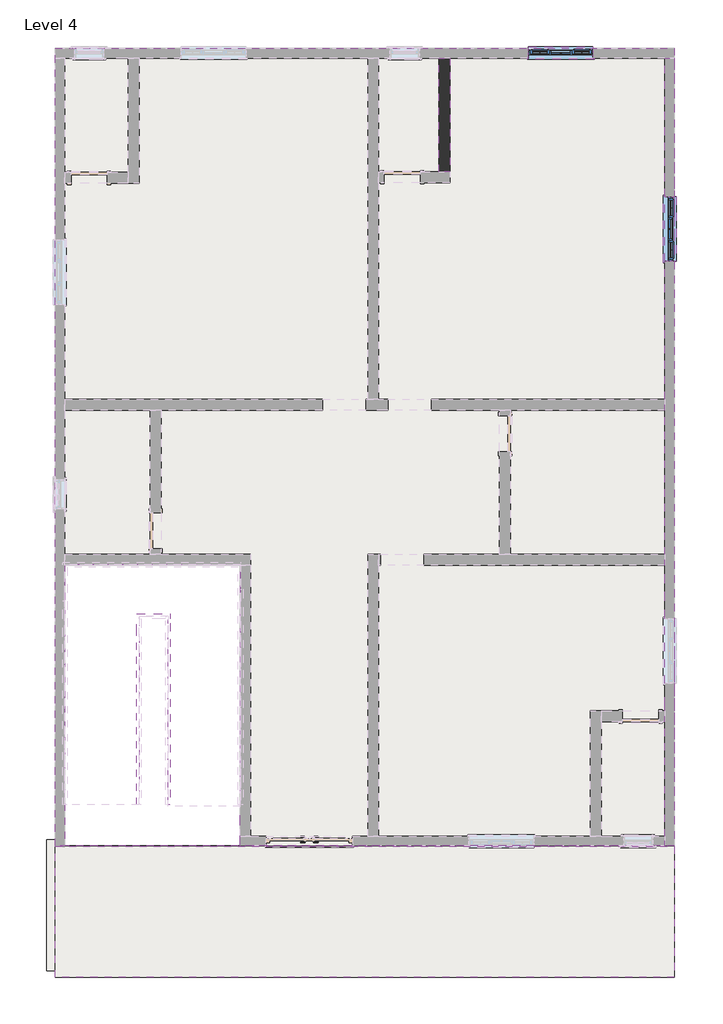
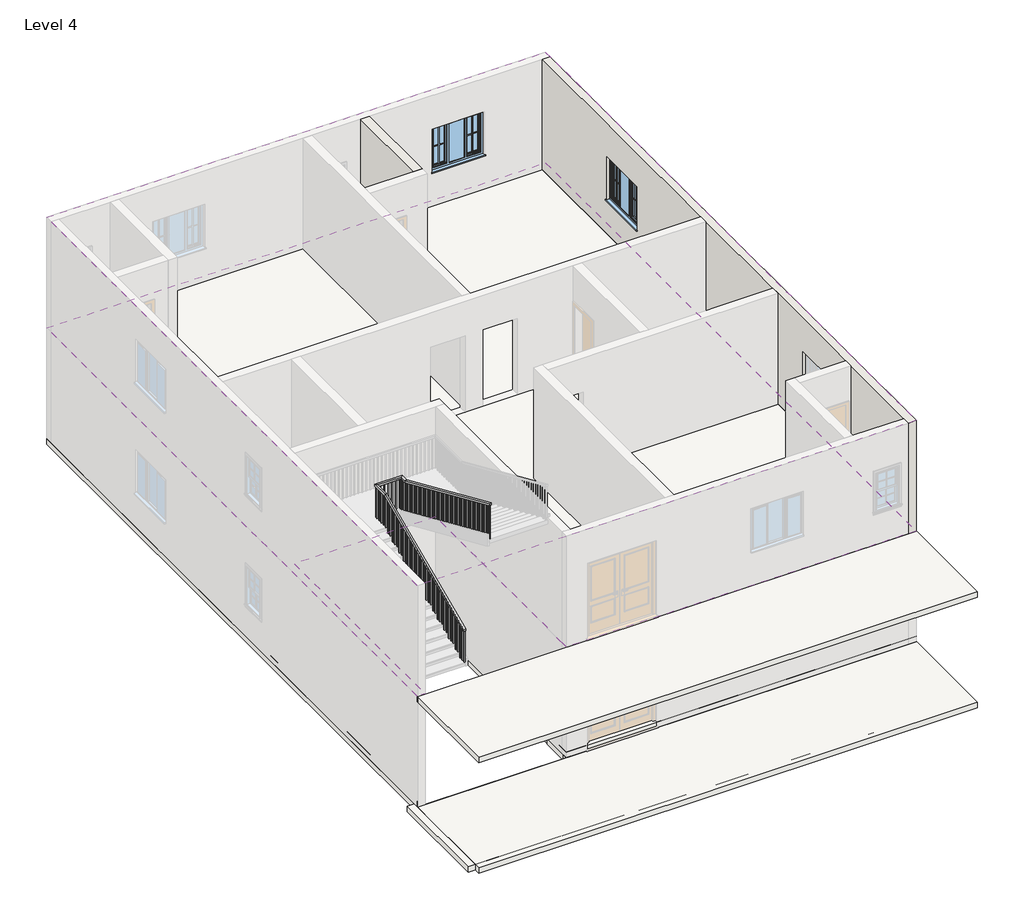
# One storey, part 3 of 5: 6 roofs, 6 slabs, 6 windows, 5 walls, 1 railing.
"""IFC4 building model written with IfcOpenShell, lengths in millimetres."""

from ifc_helpers import new_model, si_unit, frame, origin, place, context, project, spatial, polyline, outline, extrude, faceted_brep, transform, mapped, element, save
from components import windows_tpl_w_glazing_cross_bars_1360x1210mm_0306471f

model = new_model("IFC4")

# Units and contexts
model_context = context("Model", 3, world=origin())
ifc_project = project(units=[si_unit("LENGTHUNIT", "METRE", prefix="MILLI")], contexts=[model_context])

# Site, building, storey
site = spatial("IfcSite", under=ifc_project)
building = spatial("IfcBuilding", under=site)
storey = spatial("IfcBuildingStorey", under=building, Name="Level 4", Elevation=9144.0)

# Railing
placement = place(None, origin())
element("IfcRailing", 1, ObjectType="Handrail - Rectangular", at=placement, inside=storey, context=model_context, shape_type="SolidModel", body=[
    faceted_brep([(-6050.7290366, -6973.0610642, 12913.36), (-6050.7290366, -6973.0610642, 12857.8599828), (-5999.9290366, -6973.0610642, 12857.8599828), (-5999.9290366, -6973.0610642, 12913.36), (-6050.7290366, -3417.0610642, 14478.0), (-6050.7290366, -3406.3792071, 14427.2), (-5999.9290366, -3406.3792071, 14427.2), (-5999.9290366, -3417.0610642, 14478.0), (-6050.7290366, -2959.8610642, 14478.0), (-6050.7290366, -2959.8610642, 14427.2), (-5999.9290366, -3010.6610642, 14427.2), (-5999.9290366, -3010.6610642, 14478.0), (-5339.5290366, -2959.8610642, 14478.0), (-5339.5290366, -2959.8610642, 14427.2), (-5390.3290366, -3010.6610642, 14427.2), (-5390.3290366, -3010.6610642, 14478.0), (-5339.5290366, -3163.0610642, 14478.0), (-5339.5290366, -3173.7429214, 14427.2), (-5390.3290366, -3173.7429214, 14427.2), (-5390.3290366, -3163.0610642, 14478.0), (-5339.5290366, -6973.0610642, 16154.4), (-5390.3290366, -6973.0610642, 16154.4), (-5390.3290366, -6973.0610642, 16098.8999828), (-5339.5290366, -6973.0610642, 16098.8999828)], [[[0, 1, 2, 3]], [[1, 0, 4, 5]], [[2, 1, 5, 6]], [[3, 2, 6, 7]], [[0, 3, 7, 4]], [[5, 4, 8, 9]], [[6, 5, 9, 10]], [[7, 6, 10, 11]], [[4, 7, 11, 8]], [[9, 8, 12, 13]], [[10, 9, 13, 14]], [[11, 10, 14, 15]], [[8, 11, 15, 12]], [[13, 12, 16, 17]], [[14, 13, 17, 18]], [[15, 14, 18, 19]], [[12, 15, 19, 16]], [[20, 21, 22, 23]], [[17, 16, 20, 23]], [[18, 17, 23, 22]], [[19, 18, 22, 21]], [[16, 19, 21, 20]]]),
    extrude(outline(polyline([(-6957.1860642, 16091.9149828), (-6938.1360642, 16083.5329828), (-6938.1360642, 15128.24), (-6957.1860642, 15128.24), (-6957.1860642, 16091.9149828)])), frame((-5374.4540366, 0.0, 0.0), z_axis=(1.0, 0.0, 0.0), x_axis=(0.0, 1.0, 0.0)), (0.0, 0.0, 1.0), 19.05),
    extrude(outline(polyline([(-6855.5860642, 16047.2109828), (-6836.5360642, 16038.8289828), (-6836.5360642, 15128.24), (-6855.5860642, 15128.24), (-6855.5860642, 16047.2109828)])), frame((-5374.4540366, 0.0, 0.0), z_axis=(1.0, 0.0, 0.0), x_axis=(0.0, 1.0, 0.0)), (0.0, 0.0, 1.0), 19.05),
    extrude(outline(polyline([(-6753.9860642, 16002.5069828), (-6734.9360642, 15994.1249828), (-6734.9360642, 15128.24), (-6753.9860642, 15128.24), (-6753.9860642, 16002.5069828)])), frame((-5374.4540366, 0.0, 0.0), z_axis=(1.0, 0.0, 0.0), x_axis=(0.0, 1.0, 0.0)), (0.0, 0.0, 1.0), 19.05),
    extrude(outline(polyline([(-6652.3860642, 15957.8029828), (-6633.3360642, 15949.4209828), (-6633.3360642, 15016.48), (-6652.3860642, 15016.48), (-6652.3860642, 15957.8029828)])), frame((-5374.4540366, 0.0, 0.0), z_axis=(1.0, 0.0, 0.0), x_axis=(0.0, 1.0, 0.0)), (0.0, 0.0, 1.0), 19.05),
    extrude(outline(polyline([(-6550.7860642, 15913.0989828), (-6531.7360642, 15904.7169828), (-6531.7360642, 15016.48), (-6550.7860642, 15016.48), (-6550.7860642, 15913.0989828)])), frame((-5374.4540366, 0.0, 0.0), z_axis=(1.0, 0.0, 0.0), x_axis=(0.0, 1.0, 0.0)), (0.0, 0.0, 1.0), 19.05),
    extrude(outline(polyline([(-6449.1860642, 15868.3949828), (-6430.1360642, 15860.0129828), (-6430.1360642, 14904.72), (-6449.1860642, 14904.72), (-6449.1860642, 15868.3949828)])), frame((-5374.4540366, 0.0, 0.0), z_axis=(1.0, 0.0, 0.0), x_axis=(0.0, 1.0, 0.0)), (0.0, 0.0, 1.0), 19.05),
    extrude(outline(polyline([(-6347.5860642, 15823.6909828), (-6328.5360642, 15815.3089828), (-6328.5360642, 14904.72), (-6347.5860642, 14904.72), (-6347.5860642, 15823.6909828)])), frame((-5374.4540366, 0.0, 0.0), z_axis=(1.0, 0.0, 0.0), x_axis=(0.0, 1.0, 0.0)), (0.0, 0.0, 1.0), 19.05),
    extrude(outline(polyline([(-6245.9860642, 15778.9869828), (-6226.9360642, 15770.6049828), (-6226.9360642, 14904.72), (-6245.9860642, 14904.72), (-6245.9860642, 15778.9869828)])), frame((-5374.4540366, 0.0, 0.0), z_axis=(1.0, 0.0, 0.0), x_axis=(0.0, 1.0, 0.0)), (0.0, 0.0, 1.0), 19.05),
    extrude(outline(polyline([(-6144.3860642, 15734.2829828), (-6125.3360642, 15725.9009828), (-6125.3360642, 14792.96), (-6144.3860642, 14792.96), (-6144.3860642, 15734.2829828)])), frame((-5374.4540366, 0.0, 0.0), z_axis=(1.0, 0.0, 0.0), x_axis=(0.0, 1.0, 0.0)), (0.0, 0.0, 1.0), 19.05),
    extrude(outline(polyline([(-6042.7860642, 15689.5789828), (-6023.7360642, 15681.1969828), (-6023.7360642, 14792.96), (-6042.7860642, 14792.96), (-6042.7860642, 15689.5789828)])), frame((-5374.4540366, 0.0, 0.0), z_axis=(1.0, 0.0, 0.0), x_axis=(0.0, 1.0, 0.0)), (0.0, 0.0, 1.0), 19.05),
    extrude(outline(polyline([(-5941.1860642, 15644.8749828), (-5922.1360642, 15636.4929828), (-5922.1360642, 14681.2), (-5941.1860642, 14681.2), (-5941.1860642, 15644.8749828)])), frame((-5374.4540366, 0.0, 0.0), z_axis=(1.0, 0.0, 0.0), x_axis=(0.0, 1.0, 0.0)), (0.0, 0.0, 1.0), 19.05),
    extrude(outline(polyline([(-5839.5860642, 15600.1709828), (-5820.5360642, 15591.7889828), (-5820.5360642, 14681.2), (-5839.5860642, 14681.2), (-5839.5860642, 15600.1709828)])), frame((-5374.4540366, 0.0, 0.0), z_axis=(1.0, 0.0, 0.0), x_axis=(0.0, 1.0, 0.0)), (0.0, 0.0, 1.0), 19.05),
    extrude(outline(polyline([(-5737.9860642, 15555.4669828), (-5718.9360642, 15547.0849828), (-5718.9360642, 14681.2), (-5737.9860642, 14681.2), (-5737.9860642, 15555.4669828)])), frame((-5374.4540366, 0.0, 0.0), z_axis=(1.0, 0.0, 0.0), x_axis=(0.0, 1.0, 0.0)), (0.0, 0.0, 1.0), 19.05),
    extrude(outline(polyline([(-5636.3860642, 15510.7629828), (-5617.3360642, 15502.3809828), (-5617.3360642, 14569.44), (-5636.3860642, 14569.44), (-5636.3860642, 15510.7629828)])), frame((-5374.4540366, 0.0, 0.0), z_axis=(1.0, 0.0, 0.0), x_axis=(0.0, 1.0, 0.0)), (0.0, 0.0, 1.0), 19.05),
    extrude(outline(polyline([(-5534.7860642, 15466.0589828), (-5515.7360642, 15457.6769828), (-5515.7360642, 14569.44), (-5534.7860642, 14569.44), (-5534.7860642, 15466.0589828)])), frame((-5374.4540366, 0.0, 0.0), z_axis=(1.0, 0.0, 0.0), x_axis=(0.0, 1.0, 0.0)), (0.0, 0.0, 1.0), 19.05),
    extrude(outline(polyline([(-5433.1860642, 15421.3549828), (-5414.1360642, 15412.9729828), (-5414.1360642, 14457.68), (-5433.1860642, 14457.68), (-5433.1860642, 15421.3549828)])), frame((-5374.4540366, 0.0, 0.0), z_axis=(1.0, 0.0, 0.0), x_axis=(0.0, 1.0, 0.0)), (0.0, 0.0, 1.0), 19.05),
    extrude(outline(polyline([(-5331.5860642, 15376.6509828), (-5312.5360642, 15368.2689828), (-5312.5360642, 14457.68), (-5331.5860642, 14457.68), (-5331.5860642, 15376.6509828)])), frame((-5374.4540366, 0.0, 0.0), z_axis=(1.0, 0.0, 0.0), x_axis=(0.0, 1.0, 0.0)), (0.0, 0.0, 1.0), 19.05),
    extrude(outline(polyline([(-5229.9860642, 15331.9469828), (-5210.9360642, 15323.5649828), (-5210.9360642, 14457.68), (-5229.9860642, 14457.68), (-5229.9860642, 15331.9469828)])), frame((-5374.4540366, 0.0, 0.0), z_axis=(1.0, 0.0, 0.0), x_axis=(0.0, 1.0, 0.0)), (0.0, 0.0, 1.0), 19.05),
    extrude(outline(polyline([(-5128.3860642, 15287.2429828), (-5109.3360642, 15278.8609828), (-5109.3360642, 14345.92), (-5128.3860642, 14345.92), (-5128.3860642, 15287.2429828)])), frame((-5374.4540366, 0.0, 0.0), z_axis=(1.0, 0.0, 0.0), x_axis=(0.0, 1.0, 0.0)), (0.0, 0.0, 1.0), 19.05),
    extrude(outline(polyline([(-5026.7860642, 15242.5389828), (-5007.7360642, 15234.1569828), (-5007.7360642, 14345.92), (-5026.7860642, 14345.92), (-5026.7860642, 15242.5389828)])), frame((-5374.4540366, 0.0, 0.0), z_axis=(1.0, 0.0, 0.0), x_axis=(0.0, 1.0, 0.0)), (0.0, 0.0, 1.0), 19.05),
    extrude(outline(polyline([(-4925.1860642, 15197.8349828), (-4906.1360642, 15189.4529828), (-4906.1360642, 14234.16), (-4925.1860642, 14234.16), (-4925.1860642, 15197.8349828)])), frame((-5374.4540366, 0.0, 0.0), z_axis=(1.0, 0.0, 0.0), x_axis=(0.0, 1.0, 0.0)), (0.0, 0.0, 1.0), 19.05),
    extrude(outline(polyline([(-4823.5860642, 15153.1309828), (-4804.5360642, 15144.7489828), (-4804.5360642, 14234.16), (-4823.5860642, 14234.16), (-4823.5860642, 15153.1309828)])), frame((-5374.4540366, 0.0, 0.0), z_axis=(1.0, 0.0, 0.0), x_axis=(0.0, 1.0, 0.0)), (0.0, 0.0, 1.0), 19.05),
    extrude(outline(polyline([(-4721.9860642, 15108.4269828), (-4702.9360642, 15100.0449828), (-4702.9360642, 14234.16), (-4721.9860642, 14234.16), (-4721.9860642, 15108.4269828)])), frame((-5374.4540366, 0.0, 0.0), z_axis=(1.0, 0.0, 0.0), x_axis=(0.0, 1.0, 0.0)), (0.0, 0.0, 1.0), 19.05),
    extrude(outline(polyline([(-4620.3860642, 15063.7229828), (-4601.3360642, 15055.3409828), (-4601.3360642, 14122.4), (-4620.3860642, 14122.4), (-4620.3860642, 15063.7229828)])), frame((-5374.4540366, 0.0, 0.0), z_axis=(1.0, 0.0, 0.0), x_axis=(0.0, 1.0, 0.0)), (0.0, 0.0, 1.0), 19.05),
    extrude(outline(polyline([(-4518.7860642, 15019.0189828), (-4499.7360642, 15010.6369828), (-4499.7360642, 14122.4), (-4518.7860642, 14122.4), (-4518.7860642, 15019.0189828)])), frame((-5374.4540366, 0.0, 0.0), z_axis=(1.0, 0.0, 0.0), x_axis=(0.0, 1.0, 0.0)), (0.0, 0.0, 1.0), 19.05),
    extrude(outline(polyline([(-4417.1860642, 14974.3149828), (-4398.1360642, 14965.9329828), (-4398.1360642, 14010.64), (-4417.1860642, 14010.64), (-4417.1860642, 14974.3149828)])), frame((-5374.4540366, 0.0, 0.0), z_axis=(1.0, 0.0, 0.0), x_axis=(0.0, 1.0, 0.0)), (0.0, 0.0, 1.0), 19.05),
    extrude(outline(polyline([(-4315.5860642, 14929.6109828), (-4296.5360642, 14921.2289828), (-4296.5360642, 14010.64), (-4315.5860642, 14010.64), (-4315.5860642, 14929.6109828)])), frame((-5374.4540366, 0.0, 0.0), z_axis=(1.0, 0.0, 0.0), x_axis=(0.0, 1.0, 0.0)), (0.0, 0.0, 1.0), 19.05),
    extrude(outline(polyline([(-4213.9860642, 14884.9069828), (-4194.9360642, 14876.5249828), (-4194.9360642, 14010.64), (-4213.9860642, 14010.64), (-4213.9860642, 14884.9069828)])), frame((-5374.4540366, 0.0, 0.0), z_axis=(1.0, 0.0, 0.0), x_axis=(0.0, 1.0, 0.0)), (0.0, 0.0, 1.0), 19.05),
    extrude(outline(polyline([(-4112.3860642, 14840.2029828), (-4093.3360642, 14831.8209828), (-4093.3360642, 13898.88), (-4112.3860642, 13898.88), (-4112.3860642, 14840.2029828)])), frame((-5374.4540366, 0.0, 0.0), z_axis=(1.0, 0.0, 0.0), x_axis=(0.0, 1.0, 0.0)), (0.0, 0.0, 1.0), 19.05),
    extrude(outline(polyline([(-4010.7860642, 14795.4989828), (-3991.7360642, 14787.1169828), (-3991.7360642, 13898.88), (-4010.7860642, 13898.88), (-4010.7860642, 14795.4989828)])), frame((-5374.4540366, 0.0, 0.0), z_axis=(1.0, 0.0, 0.0), x_axis=(0.0, 1.0, 0.0)), (0.0, 0.0, 1.0), 19.05),
    extrude(outline(polyline([(-3909.1860642, 14750.7949828), (-3890.1360642, 14742.4129828), (-3890.1360642, 13787.12), (-3909.1860642, 13787.12), (-3909.1860642, 14750.7949828)])), frame((-5374.4540366, 0.0, 0.0), z_axis=(1.0, 0.0, 0.0), x_axis=(0.0, 1.0, 0.0)), (0.0, 0.0, 1.0), 19.05),
    extrude(outline(polyline([(-3807.5860642, 14706.0909828), (-3788.5360642, 14697.7089828), (-3788.5360642, 13787.12), (-3807.5860642, 13787.12), (-3807.5860642, 14706.0909828)])), frame((-5374.4540366, 0.0, 0.0), z_axis=(1.0, 0.0, 0.0), x_axis=(0.0, 1.0, 0.0)), (0.0, 0.0, 1.0), 19.05),
    extrude(outline(polyline([(-3705.9860642, 14661.3869828), (-3686.9360642, 14653.0049828), (-3686.9360642, 13787.12), (-3705.9860642, 13787.12), (-3705.9860642, 14661.3869828)])), frame((-5374.4540366, 0.0, 0.0), z_axis=(1.0, 0.0, 0.0), x_axis=(0.0, 1.0, 0.0)), (0.0, 0.0, 1.0), 19.05),
    extrude(outline(polyline([(-3604.3860642, 14616.6829828), (-3585.3360642, 14608.3009828), (-3585.3360642, 13675.36), (-3604.3860642, 13675.36), (-3604.3860642, 14616.6829828)])), frame((-5374.4540366, 0.0, 0.0), z_axis=(1.0, 0.0, 0.0), x_axis=(0.0, 1.0, 0.0)), (0.0, 0.0, 1.0), 19.05),
    extrude(outline(polyline([(-3502.7860642, 14571.9789828), (-3483.7360642, 14563.5969828), (-3483.7360642, 13675.36), (-3502.7860642, 13675.36), (-3502.7860642, 14571.9789828)])), frame((-5374.4540366, 0.0, 0.0), z_axis=(1.0, 0.0, 0.0), x_axis=(0.0, 1.0, 0.0)), (0.0, 0.0, 1.0), 19.05),
    extrude(outline(polyline([(-3401.1860642, 14527.2749828), (-3382.1360642, 14518.8929828), (-3382.1360642, 13563.6), (-3401.1860642, 13563.6), (-3401.1860642, 14527.2749828)])), frame((-5374.4540366, 0.0, 0.0), z_axis=(1.0, 0.0, 0.0), x_axis=(0.0, 1.0, 0.0)), (0.0, 0.0, 1.0), 19.05),
    extrude(outline(polyline([(-3299.5860642, 14482.5709828), (-3280.5360642, 14474.1889828), (-3280.5360642, 13563.6), (-3299.5860642, 13563.6), (-3299.5860642, 14482.5709828)])), frame((-5374.4540366, 0.0, 0.0), z_axis=(1.0, 0.0, 0.0), x_axis=(0.0, 1.0, 0.0)), (0.0, 0.0, 1.0), 19.05),
    extrude(outline(polyline([(-3197.9860642, 14437.8669828), (-3178.9360642, 14429.4849828), (-3178.9360642, 13563.6), (-3197.9860642, 13563.6), (-3197.9860642, 14437.8669828)])), frame((-5374.4540366, 0.0, 0.0), z_axis=(1.0, 0.0, 0.0), x_axis=(0.0, 1.0, 0.0)), (0.0, 0.0, 1.0), 19.05),
    extrude(outline(polyline([(-5374.4540366, -3077.3360642), (-5355.4040366, -3077.3360642), (-5355.4040366, -3096.3860642), (-5374.4540366, -3096.3860642), (-5374.4540366, -3077.3360642)])), frame((0.0, 0.0, 13563.6), z_axis=(0.0, 0.0, 1.0), x_axis=(1.0, 0.0, 0.0)), (0.0, 0.0, 1.0), 863.6),
    extrude(outline(polyline([(-5425.2540366, -2994.7860642), (-5425.2540366, -2975.7360642), (-5406.2040366, -2975.7360642), (-5406.2040366, -2994.7860642), (-5425.2540366, -2994.7860642)])), frame((0.0, 0.0, 13563.6), z_axis=(0.0, 0.0, 1.0), x_axis=(1.0, 0.0, 0.0)), (0.0, 0.0, 1.0), 863.6),
    extrude(outline(polyline([(-5526.8540366, -2994.7860642), (-5526.8540366, -2975.7360642), (-5507.8040366, -2975.7360642), (-5507.8040366, -2994.7860642), (-5526.8540366, -2994.7860642)])), frame((0.0, 0.0, 13563.6), z_axis=(0.0, 0.0, 1.0), x_axis=(1.0, 0.0, 0.0)), (0.0, 0.0, 1.0), 863.6),
    extrude(outline(polyline([(-5628.4540366, -2994.7860642), (-5628.4540366, -2975.7360642), (-5609.4040366, -2975.7360642), (-5609.4040366, -2994.7860642), (-5628.4540366, -2994.7860642)])), frame((0.0, 0.0, 13563.6), z_axis=(0.0, 0.0, 1.0), x_axis=(1.0, 0.0, 0.0)), (0.0, 0.0, 1.0), 863.6),
    extrude(outline(polyline([(-5730.0540366, -2994.7860642), (-5730.0540366, -2975.7360642), (-5711.0040366, -2975.7360642), (-5711.0040366, -2994.7860642), (-5730.0540366, -2994.7860642)])), frame((0.0, 0.0, 13563.6), z_axis=(0.0, 0.0, 1.0), x_axis=(1.0, 0.0, 0.0)), (0.0, 0.0, 1.0), 863.6),
    extrude(outline(polyline([(-5831.6540366, -2994.7860642), (-5831.6540366, -2975.7360642), (-5812.6040366, -2975.7360642), (-5812.6040366, -2994.7860642), (-5831.6540366, -2994.7860642)])), frame((0.0, 0.0, 13563.6), z_axis=(0.0, 0.0, 1.0), x_axis=(1.0, 0.0, 0.0)), (0.0, 0.0, 1.0), 863.6),
    extrude(outline(polyline([(-5933.2540366, -2994.7860642), (-5933.2540366, -2975.7360642), (-5914.2040366, -2975.7360642), (-5914.2040366, -2994.7860642), (-5933.2540366, -2994.7860642)])), frame((0.0, 0.0, 13563.6), z_axis=(0.0, 0.0, 1.0), x_axis=(1.0, 0.0, 0.0)), (0.0, 0.0, 1.0), 863.6),
    extrude(outline(polyline([(-6015.8040366, -3020.1860642), (-6034.8540366, -3020.1860642), (-6034.8540366, -3001.1360642), (-6015.8040366, -3001.1360642), (-6015.8040366, -3020.1860642)])), frame((0.0, 0.0, 13563.6), z_axis=(0.0, 0.0, 1.0), x_axis=(1.0, 0.0, 0.0)), (0.0, 0.0, 1.0), 863.6),
    extrude(outline(polyline([(-6015.8040366, -3121.7860642), (-6034.8540366, -3121.7860642), (-6034.8540366, -3102.7360642), (-6015.8040366, -3102.7360642), (-6015.8040366, -3121.7860642)])), frame((0.0, 0.0, 13563.6), z_axis=(0.0, 0.0, 1.0), x_axis=(1.0, 0.0, 0.0)), (0.0, 0.0, 1.0), 863.6),
    extrude(outline(polyline([(-6015.8040366, -3223.3860642), (-6034.8540366, -3223.3860642), (-6034.8540366, -3204.3360642), (-6015.8040366, -3204.3360642), (-6015.8040366, -3223.3860642)])), frame((0.0, 0.0, 13563.6), z_axis=(0.0, 0.0, 1.0), x_axis=(1.0, 0.0, 0.0)), (0.0, 0.0, 1.0), 863.6),
    extrude(outline(polyline([(-6015.8040366, -3324.9860642), (-6034.8540366, -3324.9860642), (-6034.8540366, -3305.9360642), (-6015.8040366, -3305.9360642), (-6015.8040366, -3324.9860642)])), frame((0.0, 0.0, 13563.6), z_axis=(0.0, 0.0, 1.0), x_axis=(1.0, 0.0, 0.0)), (0.0, 0.0, 1.0), 863.6),
    extrude(outline(polyline([(-3426.5860642, 14418.3089828), (-3407.5360642, 14426.6909828), (-3407.5360642, 13563.6), (-3426.5860642, 13563.6), (-3426.5860642, 14418.3089828)])), frame((-6034.8540366, 0.0, 0.0), z_axis=(1.0, 0.0, 0.0), x_axis=(0.0, 1.0, 0.0)), (0.0, 0.0, 1.0), 19.05),
    extrude(outline(polyline([(-3528.1860642, 14373.6049828), (-3509.1360642, 14381.9869828), (-3509.1360642, 13451.84), (-3528.1860642, 13451.84), (-3528.1860642, 14373.6049828)])), frame((-6034.8540366, 0.0, 0.0), z_axis=(1.0, 0.0, 0.0), x_axis=(0.0, 1.0, 0.0)), (0.0, 0.0, 1.0), 19.05),
    extrude(outline(polyline([(-3629.7860642, 14328.9009828), (-3610.7360642, 14337.2829828), (-3610.7360642, 13451.84), (-3629.7860642, 13451.84), (-3629.7860642, 14328.9009828)])), frame((-6034.8540366, 0.0, 0.0), z_axis=(1.0, 0.0, 0.0), x_axis=(0.0, 1.0, 0.0)), (0.0, 0.0, 1.0), 19.05),
    extrude(outline(polyline([(-3731.3860642, 14284.1969828), (-3712.3360642, 14292.5789828), (-3712.3360642, 13340.08), (-3731.3860642, 13340.08), (-3731.3860642, 14284.1969828)])), frame((-6034.8540366, 0.0, 0.0), z_axis=(1.0, 0.0, 0.0), x_axis=(0.0, 1.0, 0.0)), (0.0, 0.0, 1.0), 19.05),
    extrude(outline(polyline([(-3832.9860642, 14239.4929828), (-3813.9360642, 14247.8749828), (-3813.9360642, 13340.08), (-3832.9860642, 13340.08), (-3832.9860642, 14239.4929828)])), frame((-6034.8540366, 0.0, 0.0), z_axis=(1.0, 0.0, 0.0), x_axis=(0.0, 1.0, 0.0)), (0.0, 0.0, 1.0), 19.05),
    extrude(outline(polyline([(-3934.5860642, 14194.7889828), (-3915.5360642, 14203.1709828), (-3915.5360642, 13340.08), (-3934.5860642, 13340.08), (-3934.5860642, 14194.7889828)])), frame((-6034.8540366, 0.0, 0.0), z_axis=(1.0, 0.0, 0.0), x_axis=(0.0, 1.0, 0.0)), (0.0, 0.0, 1.0), 19.05),
    extrude(outline(polyline([(-4036.1860642, 14150.0849828), (-4017.1360642, 14158.4669828), (-4017.1360642, 13228.32), (-4036.1860642, 13228.32), (-4036.1860642, 14150.0849828)])), frame((-6034.8540366, 0.0, 0.0), z_axis=(1.0, 0.0, 0.0), x_axis=(0.0, 1.0, 0.0)), (0.0, 0.0, 1.0), 19.05),
    extrude(outline(polyline([(-4137.7860642, 14105.3809828), (-4118.7360642, 14113.7629828), (-4118.7360642, 13228.32), (-4137.7860642, 13228.32), (-4137.7860642, 14105.3809828)])), frame((-6034.8540366, 0.0, 0.0), z_axis=(1.0, 0.0, 0.0), x_axis=(0.0, 1.0, 0.0)), (0.0, 0.0, 1.0), 19.05),
    extrude(outline(polyline([(-4239.3860642, 14060.6769828), (-4220.3360642, 14069.0589828), (-4220.3360642, 13116.56), (-4239.3860642, 13116.56), (-4239.3860642, 14060.6769828)])), frame((-6034.8540366, 0.0, 0.0), z_axis=(1.0, 0.0, 0.0), x_axis=(0.0, 1.0, 0.0)), (0.0, 0.0, 1.0), 19.05),
    extrude(outline(polyline([(-4340.9860642, 14015.9729828), (-4321.9360642, 14024.3549828), (-4321.9360642, 13116.56), (-4340.9860642, 13116.56), (-4340.9860642, 14015.9729828)])), frame((-6034.8540366, 0.0, 0.0), z_axis=(1.0, 0.0, 0.0), x_axis=(0.0, 1.0, 0.0)), (0.0, 0.0, 1.0), 19.05),
    extrude(outline(polyline([(-4442.5860642, 13971.2689828), (-4423.5360642, 13979.6509828), (-4423.5360642, 13116.56), (-4442.5860642, 13116.56), (-4442.5860642, 13971.2689828)])), frame((-6034.8540366, 0.0, 0.0), z_axis=(1.0, 0.0, 0.0), x_axis=(0.0, 1.0, 0.0)), (0.0, 0.0, 1.0), 19.05),
    extrude(outline(polyline([(-4544.1860642, 13926.5649828), (-4525.1360642, 13934.9469828), (-4525.1360642, 13004.8), (-4544.1860642, 13004.8), (-4544.1860642, 13926.5649828)])), frame((-6034.8540366, 0.0, 0.0), z_axis=(1.0, 0.0, 0.0), x_axis=(0.0, 1.0, 0.0)), (0.0, 0.0, 1.0), 19.05),
    extrude(outline(polyline([(-4645.7860642, 13881.8609828), (-4626.7360642, 13890.2429828), (-4626.7360642, 13004.8), (-4645.7860642, 13004.8), (-4645.7860642, 13881.8609828)])), frame((-6034.8540366, 0.0, 0.0), z_axis=(1.0, 0.0, 0.0), x_axis=(0.0, 1.0, 0.0)), (0.0, 0.0, 1.0), 19.05),
    extrude(outline(polyline([(-4747.3860642, 13837.1569828), (-4728.3360642, 13845.5389828), (-4728.3360642, 12893.04), (-4747.3860642, 12893.04), (-4747.3860642, 13837.1569828)])), frame((-6034.8540366, 0.0, 0.0), z_axis=(1.0, 0.0, 0.0), x_axis=(0.0, 1.0, 0.0)), (0.0, 0.0, 1.0), 19.05),
    extrude(outline(polyline([(-4848.9860642, 13792.4529828), (-4829.9360642, 13800.8349828), (-4829.9360642, 12893.04), (-4848.9860642, 12893.04), (-4848.9860642, 13792.4529828)])), frame((-6034.8540366, 0.0, 0.0), z_axis=(1.0, 0.0, 0.0), x_axis=(0.0, 1.0, 0.0)), (0.0, 0.0, 1.0), 19.05),
    extrude(outline(polyline([(-4950.5860642, 13747.7489828), (-4931.5360642, 13756.1309828), (-4931.5360642, 12893.04), (-4950.5860642, 12893.04), (-4950.5860642, 13747.7489828)])), frame((-6034.8540366, 0.0, 0.0), z_axis=(1.0, 0.0, 0.0), x_axis=(0.0, 1.0, 0.0)), (0.0, 0.0, 1.0), 19.05),
    extrude(outline(polyline([(-5052.1860642, 13703.0449828), (-5033.1360642, 13711.4269828), (-5033.1360642, 12781.28), (-5052.1860642, 12781.28), (-5052.1860642, 13703.0449828)])), frame((-6034.8540366, 0.0, 0.0), z_axis=(1.0, 0.0, 0.0), x_axis=(0.0, 1.0, 0.0)), (0.0, 0.0, 1.0), 19.05),
    extrude(outline(polyline([(-5153.7860642, 13658.3409828), (-5134.7360642, 13666.7229828), (-5134.7360642, 12781.28), (-5153.7860642, 12781.28), (-5153.7860642, 13658.3409828)])), frame((-6034.8540366, 0.0, 0.0), z_axis=(1.0, 0.0, 0.0), x_axis=(0.0, 1.0, 0.0)), (0.0, 0.0, 1.0), 19.05),
    extrude(outline(polyline([(-5255.3860642, 13613.6369828), (-5236.3360642, 13622.0189828), (-5236.3360642, 12669.52), (-5255.3860642, 12669.52), (-5255.3860642, 13613.6369828)])), frame((-6034.8540366, 0.0, 0.0), z_axis=(1.0, 0.0, 0.0), x_axis=(0.0, 1.0, 0.0)), (0.0, 0.0, 1.0), 19.05),
    extrude(outline(polyline([(-5356.9860642, 13568.9329828), (-5337.9360642, 13577.3149828), (-5337.9360642, 12669.52), (-5356.9860642, 12669.52), (-5356.9860642, 13568.9329828)])), frame((-6034.8540366, 0.0, 0.0), z_axis=(1.0, 0.0, 0.0), x_axis=(0.0, 1.0, 0.0)), (0.0, 0.0, 1.0), 19.05),
    extrude(outline(polyline([(-5458.5860642, 13524.2289828), (-5439.5360642, 13532.6109828), (-5439.5360642, 12669.52), (-5458.5860642, 12669.52), (-5458.5860642, 13524.2289828)])), frame((-6034.8540366, 0.0, 0.0), z_axis=(1.0, 0.0, 0.0), x_axis=(0.0, 1.0, 0.0)), (0.0, 0.0, 1.0), 19.05),
    extrude(outline(polyline([(-5560.1860642, 13479.5249828), (-5541.1360642, 13487.9069828), (-5541.1360642, 12557.76), (-5560.1860642, 12557.76), (-5560.1860642, 13479.5249828)])), frame((-6034.8540366, 0.0, 0.0), z_axis=(1.0, 0.0, 0.0), x_axis=(0.0, 1.0, 0.0)), (0.0, 0.0, 1.0), 19.05),
    extrude(outline(polyline([(-5661.7860642, 13434.8209828), (-5642.7360642, 13443.2029828), (-5642.7360642, 12557.76), (-5661.7860642, 12557.76), (-5661.7860642, 13434.8209828)])), frame((-6034.8540366, 0.0, 0.0), z_axis=(1.0, 0.0, 0.0), x_axis=(0.0, 1.0, 0.0)), (0.0, 0.0, 1.0), 19.05),
    extrude(outline(polyline([(-5763.3860642, 13390.1169828), (-5744.3360642, 13398.4989828), (-5744.3360642, 12446.0), (-5763.3860642, 12446.0), (-5763.3860642, 13390.1169828)])), frame((-6034.8540366, 0.0, 0.0), z_axis=(1.0, 0.0, 0.0), x_axis=(0.0, 1.0, 0.0)), (0.0, 0.0, 1.0), 19.05),
    extrude(outline(polyline([(-5864.9860642, 13345.4129828), (-5845.9360642, 13353.7949828), (-5845.9360642, 12446.0), (-5864.9860642, 12446.0), (-5864.9860642, 13345.4129828)])), frame((-6034.8540366, 0.0, 0.0), z_axis=(1.0, 0.0, 0.0), x_axis=(0.0, 1.0, 0.0)), (0.0, 0.0, 1.0), 19.05),
    extrude(outline(polyline([(-5966.5860642, 13300.7089828), (-5947.5360642, 13309.0909828), (-5947.5360642, 12446.0), (-5966.5860642, 12446.0), (-5966.5860642, 13300.7089828)])), frame((-6034.8540366, 0.0, 0.0), z_axis=(1.0, 0.0, 0.0), x_axis=(0.0, 1.0, 0.0)), (0.0, 0.0, 1.0), 19.05),
    extrude(outline(polyline([(-6068.1860642, 13256.0049828), (-6049.1360642, 13264.3869828), (-6049.1360642, 12334.24), (-6068.1860642, 12334.24), (-6068.1860642, 13256.0049828)])), frame((-6034.8540366, 0.0, 0.0), z_axis=(1.0, 0.0, 0.0), x_axis=(0.0, 1.0, 0.0)), (0.0, 0.0, 1.0), 19.05),
    extrude(outline(polyline([(-6169.7860642, 13211.3009828), (-6150.7360642, 13219.6829828), (-6150.7360642, 12334.24), (-6169.7860642, 12334.24), (-6169.7860642, 13211.3009828)])), frame((-6034.8540366, 0.0, 0.0), z_axis=(1.0, 0.0, 0.0), x_axis=(0.0, 1.0, 0.0)), (0.0, 0.0, 1.0), 19.05),
    extrude(outline(polyline([(-6271.3860642, 13166.5969828), (-6252.3360642, 13174.9789828), (-6252.3360642, 12222.48), (-6271.3860642, 12222.48), (-6271.3860642, 13166.5969828)])), frame((-6034.8540366, 0.0, 0.0), z_axis=(1.0, 0.0, 0.0), x_axis=(0.0, 1.0, 0.0)), (0.0, 0.0, 1.0), 19.05),
    extrude(outline(polyline([(-6372.9860642, 13121.8929828), (-6353.9360642, 13130.2749828), (-6353.9360642, 12222.48), (-6372.9860642, 12222.48), (-6372.9860642, 13121.8929828)])), frame((-6034.8540366, 0.0, 0.0), z_axis=(1.0, 0.0, 0.0), x_axis=(0.0, 1.0, 0.0)), (0.0, 0.0, 1.0), 19.05),
    extrude(outline(polyline([(-6474.5860642, 13077.1889828), (-6455.5360642, 13085.5709828), (-6455.5360642, 12222.48), (-6474.5860642, 12222.48), (-6474.5860642, 13077.1889828)])), frame((-6034.8540366, 0.0, 0.0), z_axis=(1.0, 0.0, 0.0), x_axis=(0.0, 1.0, 0.0)), (0.0, 0.0, 1.0), 19.05),
    extrude(outline(polyline([(-6576.1860642, 13032.4849828), (-6557.1360642, 13040.8669828), (-6557.1360642, 12110.72), (-6576.1860642, 12110.72), (-6576.1860642, 13032.4849828)])), frame((-6034.8540366, 0.0, 0.0), z_axis=(1.0, 0.0, 0.0), x_axis=(0.0, 1.0, 0.0)), (0.0, 0.0, 1.0), 19.05),
    extrude(outline(polyline([(-6677.7860642, 12987.7809828), (-6658.7360642, 12996.1629828), (-6658.7360642, 12110.72), (-6677.7860642, 12110.72), (-6677.7860642, 12987.7809828)])), frame((-6034.8540366, 0.0, 0.0), z_axis=(1.0, 0.0, 0.0), x_axis=(0.0, 1.0, 0.0)), (0.0, 0.0, 1.0), 19.05),
    extrude(outline(polyline([(-6779.3860642, 12943.0769828), (-6760.3360642, 12951.4589828), (-6760.3360642, 11998.96), (-6779.3860642, 11998.96), (-6779.3860642, 12943.0769828)])), frame((-6034.8540366, 0.0, 0.0), z_axis=(1.0, 0.0, 0.0), x_axis=(0.0, 1.0, 0.0)), (0.0, 0.0, 1.0), 19.05),
    extrude(outline(polyline([(-6880.9860642, 12898.3729828), (-6861.9360642, 12906.7549828), (-6861.9360642, 11998.96), (-6880.9860642, 11998.96), (-6880.9860642, 12898.3729828)])), frame((-6034.8540366, 0.0, 0.0), z_axis=(1.0, 0.0, 0.0), x_axis=(0.0, 1.0, 0.0)), (0.0, 0.0, 1.0), 19.05),
    extrude(outline(polyline([(-5374.4540366, -2994.7860642), (-5374.4540366, -2975.7360642), (-5355.4040366, -2975.7360642), (-5355.4040366, -2994.7860642), (-5374.4540366, -2994.7860642)])), frame((0.0, 0.0, 13563.6), z_axis=(0.0, 0.0, 1.0), x_axis=(1.0, 0.0, 0.0)), (0.0, 0.0, 1.0), 863.6),
    extrude(outline(polyline([(-6015.8040366, -2994.7860642), (-6034.8540366, -2994.7860642), (-6034.8540366, -2975.7360642), (-6015.8040366, -2975.7360642), (-6015.8040366, -2994.7860642)])), frame((0.0, 0.0, 13563.6), z_axis=(0.0, 0.0, 1.0), x_axis=(1.0, 0.0, 0.0)), (0.0, 0.0, 1.0), 863.6),
    extrude(outline(polyline([(-6973.0610642, 16098.8999828), (-6954.0110642, 16090.5179828), (-6954.0110642, 15128.24), (-6973.0610642, 15128.24), (-6973.0610642, 16098.8999828)])), frame((-5374.4540366, 0.0, 0.0), z_axis=(1.0, 0.0, 0.0), x_axis=(0.0, 1.0, 0.0)), (0.0, 0.0, 1.0), 19.05),
    extrude(outline(polyline([(-6973.0610642, 12857.8599828), (-6954.0110642, 12866.2419828), (-6954.0110642, 11998.96), (-6973.0610642, 11998.96), (-6973.0610642, 12857.8599828)])), frame((-6034.8540366, 0.0, 0.0), z_axis=(1.0, 0.0, 0.0), x_axis=(0.0, 1.0, 0.0)), (0.0, 0.0, 1.0), 19.05),
])

# Roofs
element("IfcRoof", 2, ObjectType="Generic - 12\"", at=placement, inside=storey, context=model_context, shape_type="SweptSolid", body=[
    extrude(outline(polyline([(-7757.6415084, 8907.4935985), (5247.1584916, 8907.4935985), (5247.1584916, -7831.1064015), (-3879.0290366, -7831.1064015), (-3879.0290366, -6973.0610642), (-3866.3290366, -6973.0610642), (-3866.3290366, -1928.4217109), (-7554.4415084, -1928.4217109), (-7554.4415084, -7831.1064015), (-7757.6415084, -7831.1064015), (-7757.6415084, 8907.4935985)])), frame((0.0, 0.0, 9144.0), z_axis=(0.0, 0.0, 1.0), x_axis=(1.0, 0.0, 0.0)), (0.0, 0.0, 1.0), 152.4),
])
element("IfcRoof", 3, ObjectType="Generic - 12\"", at=placement, inside=storey, context=model_context, shape_type="SweptSolid", body=[
    extrude(outline(polyline([(-7757.6415084, 8907.4935985), (5247.1584916, 8907.4935985), (5247.1584916, -7831.1064015), (-3879.0290366, -7831.1064015), (-3879.0290366, -6973.0610642), (-3866.3290366, -6973.0610642), (-3866.3290366, -1928.4217109), (-7554.4415084, -1928.4217109), (-7554.4415084, -7831.1064015), (-7757.6415084, -7831.1064015), (-7757.6415084, 8907.4935985)])), frame((0.0, 0.0, 12192.0), z_axis=(0.0, 0.0, 1.0), x_axis=(1.0, 0.0, 0.0)), (0.0, 0.0, 1.0), 152.4),
])
element("IfcRoof", 4, ObjectType="Generic - 12\"", at=placement, inside=storey, context=model_context, shape_type="SweptSolid", body=[
    extrude(outline(polyline([(-7757.6415084, 8907.4935985), (5247.1584916, 8907.4935985), (5247.1584916, -7831.1064015), (-3879.0290366, -7831.1064015), (-3879.0290366, -6973.0610642), (-3866.3290366, -6973.0610642), (-3866.3290366, -1928.4217109), (-7554.4415084, -1928.4217109), (-7554.4415084, -7831.1064015), (-7757.6415084, -7831.1064015), (-7757.6415084, 8907.4935985)])), frame((0.0, 0.0, 12192.0), z_axis=(0.0, 0.0, 1.0), x_axis=(1.0, 0.0, 0.0)), (0.0, 0.0, 1.0), 152.4),
])
element("IfcRoof", 5, ObjectType="Generic - 12\"", at=placement, inside=storey, context=model_context, shape_type="SweptSolid", body=[
    extrude(outline(polyline([(-7757.6415084, 8907.4935985), (5247.1584916, 8907.4935985), (5247.1584916, -7831.1064015), (-3879.0290366, -7831.1064015), (-3879.0290366, -6973.0610642), (-3866.3290366, -6973.0610642), (-3866.3290366, -1928.4217109), (-7554.4415084, -1928.4217109), (-7554.4415084, -7831.1064015), (-7757.6415084, -7831.1064015), (-7757.6415084, 8907.4935985)])), frame((0.0, 0.0, 12192.0), z_axis=(0.0, 0.0, 1.0), x_axis=(1.0, 0.0, 0.0)), (0.0, 0.0, 1.0), 152.4),
])
element("IfcRoof", 6, ObjectType="Generic - 12\"", at=placement, inside=storey, context=model_context, shape_type="SweptSolid", body=[
    extrude(outline(polyline([(5247.1584916, -7831.1064015), (-7757.6415084, -7831.1064015), (-7757.6415084, 8907.4935985), (5247.1584916, 8907.4935985), (5247.1584916, -7831.1064015)]), holes=[polyline([(-3866.3290366, -1928.4217109), (-7554.4415084, -1928.4217109), (-7554.4415084, -6973.0610642), (-3866.3290366, -6973.0610642), (-3866.3290366, -1928.4217109)])]), frame((0.0, 0.0, 15240.0), z_axis=(0.0, 0.0, 1.0), x_axis=(1.0, 0.0, 0.0)), (0.0, 0.0, 1.0), 152.4),
])
element("IfcRoof", 7, ObjectType="Generic - 12\"", at=placement, inside=storey, context=model_context, shape_type="SweptSolid", body=[
    extrude(outline(polyline([(5247.1584916, -7831.1064015), (-7757.6415084, -7831.1064015), (-7757.6415084, 8907.4935985), (5247.1584916, 8907.4935985), (5247.1584916, -7831.1064015)]), holes=[polyline([(-3866.3290366, -1928.4217109), (-7554.4415084, -1928.4217109), (-7554.4415084, -6973.0610642), (-3866.3290366, -6973.0610642), (-3866.3290366, -1928.4217109)])]), frame((0.0, 0.0, 15240.0), z_axis=(0.0, 0.0, 1.0), x_axis=(1.0, 0.0, 0.0)), (0.0, 0.0, 1.0), 152.4),
])

# Slabs
element("IfcSlab", 8, ObjectType="Generic - 12\"", at=placement, inside=storey, context=model_context, shape_type="SweptSolid", body=[
    extrude(outline(polyline([(5247.1584916, 8907.4935985), (5247.1584916, -7831.1064015), (-3879.0290366, -7831.1064015), (-3879.0290366, -6973.0610642), (-3866.3290366, -6973.0610642), (-3866.3290366, -1928.4217109), (-7554.4415084, -1928.4217109), (-7554.4415084, -7831.1064015), (-7757.6415084, -7831.1064015), (-7757.6415084, 8907.4935985), (5247.1584916, 8907.4935985)])), frame((0.0, 0.0, 8991.6), z_axis=(0.0, 0.0, 1.0), x_axis=(1.0, 0.0, 0.0)), (0.0, 0.0, 1.0), 152.4),
])
element("IfcSlab", 9, ObjectType="Generic - 12\"", at=placement, inside=storey, context=model_context, shape_type="SweptSolid", body=[
    extrude(outline(polyline([(5247.1584916, -7843.8064015), (5247.1584916, -10593.3139891), (-7757.6415084, -10593.3139891), (-7757.6415084, -7843.8064015), (5247.1584916, -7843.8064015)])), frame((0.0, 0.0, 8991.6), z_axis=(0.0, 0.0, 1.0), x_axis=(1.0, 0.0, 0.0)), (0.0, 0.0, 1.0), 152.4),
])
element("IfcSlab", 10, ObjectType="Generic - 12\"", at=placement, inside=storey, context=model_context, shape_type="SweptSolid", body=[
    extrude(outline(polyline([(5247.1584916, 8907.4935985), (5247.1584916, -7831.1064015), (-3879.0290366, -7831.1064015), (-3879.0290366, -6973.0610642), (-3866.3290366, -6973.0610642), (-3866.3290366, -1928.4217109), (-7554.4415084, -1928.4217109), (-7554.4415084, -7831.1064015), (-7757.6415084, -7831.1064015), (-7757.6415084, 8907.4935985), (5247.1584916, 8907.4935985)])), frame((0.0, 0.0, 8991.6), z_axis=(0.0, 0.0, 1.0), x_axis=(1.0, 0.0, 0.0)), (0.0, 0.0, 1.0), 152.4),
])
element("IfcSlab", 11, ObjectType="Generic - 12\"", at=placement, inside=storey, context=model_context, shape_type="SweptSolid", body=[
    extrude(outline(polyline([(5247.1584916, 8907.4935985), (5247.1584916, -7831.1064015), (-3879.0290366, -7831.1064015), (-3879.0290366, -6973.0610642), (-3866.3290366, -6973.0610642), (-3866.3290366, -1928.4217109), (-7554.4415084, -1928.4217109), (-7554.4415084, -7831.1064015), (-7757.6415084, -7831.1064015), (-7757.6415084, 8907.4935985), (5247.1584916, 8907.4935985)])), frame((0.0, 0.0, 12039.6), z_axis=(0.0, 0.0, 1.0), x_axis=(1.0, 0.0, 0.0)), (0.0, 0.0, 1.0), 152.4),
])
element("IfcSlab", 12, ObjectType="Generic - 12\"", at=placement, inside=storey, context=model_context, shape_type="SweptSolid", body=[
    extrude(outline(polyline([(5063.8122085, -7701.6194881), (5063.8122085, -10451.1270757), (-7940.9877915, -10451.1270757), (-7940.9877915, -7701.6194881), (-7554.4415084, -7701.6194881), (-7554.4415084, -7831.1064015), (-3879.0290366, -7831.1064015), (-3879.0290366, -7701.6194881), (5063.8122085, -7701.6194881)])), frame((0.0, 0.0, 8991.6), z_axis=(0.0, 0.0, 1.0), x_axis=(1.0, 0.0, 0.0)), (0.0, 0.0, 1.0), 152.4),
])
element("IfcSlab", 13, ObjectType="Generic - 12\"", at=placement, inside=storey, context=model_context, shape_type="SweptSolid", body=[
    extrude(outline(polyline([(5247.1584916, -7843.8064015), (5247.1584916, -10593.3139891), (-7757.6415084, -10593.3139891), (-7757.6415084, -7843.8064015), (5247.1584916, -7843.8064015)])), frame((0.0, 0.0, 12039.6), z_axis=(0.0, 0.0, 1.0), x_axis=(1.0, 0.0, 0.0)), (0.0, 0.0, 1.0), 152.4),
])

# Walls
element("IfcWall", 14, ObjectType="Generic - 4.5\"", at=placement, inside=storey, context=model_context, shape_type="SweptSolid", body=[
    extrude(outline(polyline([(535.4584916, 8704.2935985), (535.4584916, 6317.5000968), (306.8584916, 6317.5000968), (306.8584916, 8704.2935985), (535.4584916, 8704.2935985)])), frame((0.0, 0.0, 9144.0), z_axis=(0.0, 0.0, 1.0), x_axis=(1.0, 0.0, 0.0)), (0.0, 0.0, 1.0), 3048.0),
])
element("IfcWall", 15, ObjectType="Generic - 4.5\"", at=placement, inside=storey, context=model_context, shape_type="SweptSolid", body=[
    extrude(outline(polyline([(535.4584916, 8704.2935985), (535.4584916, 6317.5000968), (306.8584916, 6317.5000968), (306.8584916, 8704.2935985), (535.4584916, 8704.2935985)])), frame((0.0, 0.0, 9144.0), z_axis=(0.0, 0.0, 1.0), x_axis=(1.0, 0.0, 0.0)), (0.0, 0.0, 1.0), 3048.0),
])
element("IfcWall", 16, ObjectType="Generic - 4.5\"", at=placement, inside=storey, context=model_context, shape_type="SweptSolid", body=[
    extrude(outline(polyline([(535.4584916, 8704.2935985), (535.4584916, 6317.5000968), (306.8584916, 6317.5000968), (306.8584916, 8704.2935985), (535.4584916, 8704.2935985)])), frame((0.0, 0.0, 12192.0), z_axis=(0.0, 0.0, 1.0), x_axis=(1.0, 0.0, 0.0)), (0.0, 0.0, 1.0), 3048.0),
])
element("IfcWall", 17, ObjectType="Generic - 9\"", at=placement, inside=storey, context=model_context, shape_type="Brep", body=[
    faceted_brep([(5043.9584916, 8704.2935985, 9144.0), (5043.9584916, 1541.4935985, 9144.0), (5043.9584916, 1312.8935985, 9144.0), (5043.9584916, -1712.5217109, 9144.0), (5043.9584916, -1941.1217109, 9144.0), (5043.9584916, -4999.0064015, 9144.0), (5043.9584916, -5227.6064015, 9144.0), (5043.9584916, -7627.9064015, 9144.0), (5043.9584916, -7627.9064015, 12192.0), (5043.9584916, -5227.6064015, 12192.0), (5043.9584916, -4999.0064015, 12192.0), (5043.9584916, -1941.1217109, 12192.0), (5043.9584916, -1712.5217109, 12192.0), (5043.9584916, 1312.8935985, 12192.0), (5043.9584916, 1541.4935985, 12192.0), (5043.9584916, 8704.2935985, 12192.0), (5043.9584916, 5796.5435985, 11268.4), (5043.9584916, 4436.5435985, 11268.4), (5043.9584916, 4436.5435985, 10058.4), (5043.9584916, 5796.5435985, 10058.4), (5043.9584916, -3061.7064015, 11268.4), (5043.9584916, -4421.7064015, 11268.4), (5043.9584916, -4421.7064015, 10058.4), (5043.9584916, -3061.7064015, 10058.4), (5247.1584916, 8704.2935985, 9144.0), (5247.1584916, 8704.2935985, 12192.0), (5247.1584916, -7627.9064015, 12192.0), (5247.1584916, -7627.9064015, 9144.0), (5247.1584916, 5796.5435985, 11268.4), (5247.1584916, 5796.5435985, 10058.4), (5247.1584916, 4436.5435985, 10058.4), (5247.1584916, 4436.5435985, 11268.4), (5247.1584916, -3061.7064015, 11268.4), (5247.1584916, -3061.7064015, 10058.4), (5247.1584916, -4421.7064015, 10058.4), (5247.1584916, -4421.7064015, 11268.4)], [[[0, 1, 2, 3, 4, 5, 6, 7, 8, 9, 10, 11, 12, 13, 14, 15], [16, 17, 18, 19], [20, 21, 22, 23]], [[24, 25, 26, 27], [28, 29, 30, 31], [32, 33, 34, 35]], [[7, 6, 5, 4, 3, 2, 1, 0, 24, 27]], [[15, 14, 13, 12, 11, 10, 9, 8, 26, 25]], [[29, 28, 16, 19]], [[30, 29, 19, 18]], [[31, 30, 18, 17]], [[28, 31, 17, 16]], [[33, 32, 20, 23]], [[34, 33, 23, 22]], [[35, 34, 22, 21]], [[32, 35, 21, 20]], [[0, 15, 25, 24]], [[8, 7, 27, 26]]]),
])
element("IfcWall", 18, ObjectType="Generic - 9\"", at=placement, inside=storey, context=model_context, shape_type="Brep", body=[
    faceted_brep([(5043.9584916, 8704.2935985, 12192.0), (5043.9584916, 1541.4935985, 12192.0), (5043.9584916, 1312.8935985, 12192.0), (5043.9584916, -1712.5217109, 12192.0), (5043.9584916, -1941.1217109, 12192.0), (5043.9584916, -4999.0064015, 12192.0), (5043.9584916, -5227.6064015, 12192.0), (5043.9584916, -7627.9064015, 12192.0), (5043.9584916, -7831.1064015, 12192.0), (5043.9584916, -7831.1064015, 15240.0), (5043.9584916, -7627.9064015, 15240.0), (5043.9584916, -5227.6064015, 15240.0), (5043.9584916, -4999.0064015, 15240.0), (5043.9584916, -1941.1217109, 15240.0), (5043.9584916, -1712.5217109, 15240.0), (5043.9584916, 1312.8935985, 15240.0), (5043.9584916, 1541.4935985, 15240.0), (5043.9584916, 8704.2935985, 15240.0), (5043.9584916, 5796.5435985, 14316.4), (5043.9584916, 4436.5435985, 14316.4), (5043.9584916, 4436.5435985, 13106.4), (5043.9584916, 5796.5435985, 13106.4), (5043.9584916, -3061.7064015, 14316.4), (5043.9584916, -4421.7064015, 14316.4), (5043.9584916, -4421.7064015, 13106.4), (5043.9584916, -3061.7064015, 13106.4), (5247.1584916, 8704.2935985, 12192.0), (5247.1584916, 8704.2935985, 15240.0), (5247.1584916, -7831.1064015, 15240.0), (5247.1584916, -7831.1064015, 12192.0), (5247.1584916, 5796.5435985, 14316.4), (5247.1584916, 5796.5435985, 13106.4), (5247.1584916, 4436.5435985, 13106.4), (5247.1584916, 4436.5435985, 14316.4), (5247.1584916, -3061.7064015, 14316.4), (5247.1584916, -3061.7064015, 13106.4), (5247.1584916, -4421.7064015, 13106.4), (5247.1584916, -4421.7064015, 14316.4)], [[[0, 1, 2, 3, 4, 5, 6, 7, 8, 9, 10, 11, 12, 13, 14, 15, 16, 17], [18, 19, 20, 21], [22, 23, 24, 25]], [[26, 27, 28, 29], [30, 31, 32, 33], [34, 35, 36, 37]], [[8, 7, 6, 5, 4, 3, 2, 1, 0, 26, 29]], [[17, 16, 15, 14, 13, 12, 11, 10, 9, 28, 27]], [[31, 30, 18, 21]], [[32, 31, 21, 20]], [[33, 32, 20, 19]], [[30, 33, 19, 18]], [[35, 34, 22, 25]], [[36, 35, 25, 24]], [[37, 36, 24, 23]], [[34, 37, 23, 22]], [[0, 17, 27, 26]], [[9, 8, 29, 28]]]),
])

# Windows
windows_tpl_w_glazing_cross_bars_1360x1210mm_shape = windows_tpl_w_glazing_cross_bars_1360x1210mm_0306471f(model_context)
element("IfcWindow", 19, ObjectType="Windows_Tpl_w-Glazing_Cross-Bars : 1360x1210mm", at=placement, inside=storey, context=model_context, shape_type="MappedRepresentation", body=[
    mapped(windows_tpl_w_glazing_cross_bars_1360x1210mm_shape, transform((5137.1019238, 4614.8769318, 9158.4), x_axis=(0.0, -1.0, 0.0), y_axis=(1.0, 0.0, 0.0), z_axis=(0.0, 0.0, 1.0))),
])
element("IfcWindow", 20, ObjectType="Windows_Tpl_w-Glazing_Cross-Bars : 1360x1210mm", at=placement, inside=storey, context=model_context, shape_type="MappedRepresentation", body=[
    mapped(windows_tpl_w_glazing_cross_bars_1360x1210mm_shape, transform((3361.2251583, 8797.4370307, 9158.4), x_axis=(1.0, 0.0, 0.0), y_axis=(0.0, 1.0, 0.0), z_axis=(0.0, 0.0, 1.0))),
])
element("IfcWindow", 21, ObjectType="Windows_Tpl_w-Glazing_Cross-Bars : 1360x1210mm", at=placement, inside=storey, context=model_context, shape_type="MappedRepresentation", body=[
    mapped(windows_tpl_w_glazing_cross_bars_1360x1210mm_shape, transform((5137.1019238, 4614.8769318, 9158.4), x_axis=(0.0, -1.0, 0.0), y_axis=(1.0, 0.0, 0.0), z_axis=(0.0, 0.0, 1.0))),
])
element("IfcWindow", 22, ObjectType="Windows_Tpl_w-Glazing_Cross-Bars : 1360x1210mm", at=placement, inside=storey, context=model_context, shape_type="MappedRepresentation", body=[
    mapped(windows_tpl_w_glazing_cross_bars_1360x1210mm_shape, transform((3361.2251583, 8797.4370307, 9158.4), x_axis=(1.0, 0.0, 0.0), y_axis=(0.0, 1.0, 0.0), z_axis=(0.0, 0.0, 1.0))),
])
element("IfcWindow", 23, ObjectType="Windows_Tpl_w-Glazing_Cross-Bars : 1360x1210mm", at=placement, inside=storey, context=model_context, shape_type="MappedRepresentation", body=[
    mapped(windows_tpl_w_glazing_cross_bars_1360x1210mm_shape, transform((5137.1019238, 4614.8769318, 12206.4), x_axis=(0.0, -1.0, 0.0), y_axis=(1.0, 0.0, 0.0), z_axis=(0.0, 0.0, 1.0))),
])
element("IfcWindow", 24, ObjectType="Windows_Tpl_w-Glazing_Cross-Bars : 1360x1210mm", at=placement, inside=storey, context=model_context, shape_type="MappedRepresentation", body=[
    mapped(windows_tpl_w_glazing_cross_bars_1360x1210mm_shape, transform((3361.2251583, 8797.4370307, 12206.4), x_axis=(1.0, 0.0, 0.0), y_axis=(0.0, 1.0, 0.0), z_axis=(0.0, 0.0, 1.0))),
])

save(model, "model.ifc")

# Revit data of these elements
# Type "Handrail - Rectangular"
#   Assembly Code = "C2010400"
#   built-in parameter 1008612 = 0.0416667 (stored number, unit not read)
#   built-in parameter 1008611 = 0.0416667 (stored number, unit not read)
#   built-in parameter 1008609 = 0.333333 (stored number, unit not read)
#   built-in parameter 1008604 = 0.166667 (stored number, unit not read)
#   built-in parameter 1008603 = 0.166667 (stored number, unit not read)
#   Railing Height = 3' - 0"
#   built-in parameter 1008630 = 2
#   built-in parameter 1008610 = 2
#   built-in parameter 1008618 = Baluster - Square : 3/4"
# Type "Generic - 12\""
#   Assembly Code = "B1020"
#   Layers, outside or top first: 0' - 6" no material (function 1)
# Type "Generic - 12\""
#   Assembly Code = "B1010"
#   Function = 0
#   Layers, outside or top first: 0' - 6" no material (function 1)
# Type "Generic - 4.5\""
#   Assembly Code = "B2010"
#   Layers, outside or top first: 0' - 9" no material (function 1)
# Type "Generic - 9\""
#   Assembly Code = "B2010"
#   Layers, outside or top first: 0' - 8" no material (function 1)
# Type "Windows_Tpl_w-Glazing_Cross-Bars : 1360x1210mm"
#   Type Mark = "21"
#   Operation = "TriplePanelVertical"
#   Construction Type Id = "GSP4R"
#   Manufacturer = "Revit"
#   Keynote = "L10"
#   Analytic Construction = "1/8 in Pilkington single glazing"
#   Wrap Layers (Ext) from Ext = 0' - 4.03543"
#   Wrap Layers (Int) from Ext = 0' - 6.98819"
#   Window Board Projection = 0' - 0.98425"
#   Window Board Extension = 0' - 0.98425"
#   Visual Light Transmittance = 0.9
#   Solar Heat Gain Coefficient = 0.78
#   Rough Width = 4' - 5.54331"
#   Rough Height = 3' - 11.6378"
#   Height = 3' - 11.6378"
#   Width = 4' - 5.54331"
#   Heat Transfer Coefficient (U) = 0.6496 BTU/(h·ft²·°F)
#   Glazing Thickness = 0' - 0.94488"
#   Glazing Bar Thickness = 0' - 0.7874"
#   FrameOffset - External = 0' - 1.9685"
#   Frame Depth = 0' - 2.55906"
#   Default Head Height = 6' - 11.07087"
#   Cill Depth = 0' - 3.44488"
#   Cavity Closer Width = 0' - 1.9685"
#   Cavity Closer Offset from Ext = 0' - 4.03543"
#   Cavity Closer Depth = 0' - 3.34646"
#   Vis - Glazing Bars = yes
#   Vis - Cavity Closers = yes
#   Define Thermal Properties by = 1
#   Material Trim = Window Frame
#   Material Glazing Bars = Window Frame
#   Material Glass = Glass
#   Material Frame = Window Frame
#   Wall Closure = (empty or 0)
# Element 1 (IfcRailing, "Handrail - Rectangular")
#   Phase Created = New Construction
# Element 2 (IfcRoof, "Generic - 12\"")
#   built-in parameter 1001705 = 30.5 (stored number, unit not read)
#   built-in parameter 1001710 = 33615
#   Phase Created = New Construction
#   Materials on its faces: "Default Roof"
# Elements 3, 4, 5 (IfcRoof, "Generic - 12\"")
#   built-in parameter 1001705 = 40.5 (stored number, unit not read)
#   built-in parameter 1001701 = 10 (stored number, unit not read)
#   built-in parameter 1001710 = 33615
#   Phase Created = New Construction
#   Materials on its faces: "Default Roof"
# Element 6 (IfcRoof, "Generic - 12\"")
#   built-in parameter 1001705 = 50.5 (stored number, unit not read)
#   built-in parameter 1001701 = 20 (stored number, unit not read)
#   built-in parameter 1001710 = 33615
#   Phase Created = New Construction
#   Materials on its faces: "Default Roof"
# Element 7 (IfcRoof, "Generic - 12\"")
#   built-in parameter 1001705 = 50.5 (stored number, unit not read)
#   built-in parameter 1001701 = 20 (stored number, unit not read)
#   built-in parameter 1001710 = 33615
#   Phase Created = New Construction
#   Materials on its faces: "Default Roof", "Concrete, Precast"
# Elements 8, 10 (IfcSlab, "Generic - 12\"")
#   Height Offset From Level = 0' - 0"
#   Phase Created = New Construction
#   Materials on its faces: "Default Floor"
# Element 9 (IfcSlab, "Generic - 12\"")
#   Height Offset From Level = 0' - 0"
#   Phase Created = New Construction
#   Materials on its faces: "Default Floor", "Default Mass Interior Wall"
# Element 11 (IfcSlab, "Generic - 12\"")
#   Height Offset From Level = 10' - 0"
#   Phase Created = New Construction
#   Materials on its faces: "Default Floor", "Bed-white fabric"
# Element 12 (IfcSlab, "Generic - 12\"")
#   Height Offset From Level = 0' - 0"
#   Phase Created = New Construction
#   Materials on its faces: "Default Floor", "Concrete, Precast"
# Element 13 (IfcSlab, "Generic - 12\"")
#   Height Offset From Level = 10' - 0"
#   Phase Created = New Construction
#   Materials on its faces: "Analytical Surface - Operable Windows", "Default Floor", "Concrete, Precast", "Default Mass Interior Wall"
# Elements 14, 15 (IfcWall, "Generic - 4.5\"")
#   Top Offset = 10' - 0"
#   Base Offset = 0' - 0"
#   wall height = 10' - 0"
#   Phase Created = New Construction
#   Base Constraint = Level 4
#   Top Constraint = Level 4
#   Materials on its faces: "Default Wall"
# Element 16 (IfcWall, "Generic - 4.5\"")
#   built-in parameter 1001111 = 10' - 0"
#   Top Offset = 20' - 0"
#   Base Offset = 10' - 0"
#   wall height = 10' - 0"
#   Phase Created = New Construction
#   Base Constraint = Level 4
#   Top Constraint = Level 4
#   Materials on its faces: "Default Wall"
# Element 17 (IfcWall, "Generic - 9\"")
#   Top Offset = 10' - 0"
#   Base Offset = 0' - 0"
#   wall height = 10' - 0"
#   Phase Created = New Construction
#   Base Constraint = Level 4
#   Top Constraint = Level 4
#   Materials on its faces: "Default Wall", "Bed-white fabric"
# Element 18 (IfcWall, "Generic - 9\"")
#   built-in parameter 1001111 = 10' - 0"
#   Top Offset = 20' - 0"
#   Base Offset = 10' - 0"
#   wall height = 10' - 0"
#   Phase Created = New Construction
#   Base Constraint = Level 4
#   Top Constraint = Level 4
#   Materials on its faces: "Default Wall", "Bed-white fabric", "Bed-red fabric"
# Element 19 (IfcWindow, "Windows_Tpl_w-Glazing_Cross-Bars : 1360x1210mm")
#   Mark = "38"
#   Phase Created = New Construction
#   Materials on its faces: "Window Frame", "Glass"
# Element 20 (IfcWindow, "Windows_Tpl_w-Glazing_Cross-Bars : 1360x1210mm")
#   Mark = "41"
#   Phase Created = New Construction
#   Materials on its faces: "Window Frame", "Glass"
# Element 21 (IfcWindow, "Windows_Tpl_w-Glazing_Cross-Bars : 1360x1210mm")
#   Mark = "48"
#   Phase Created = New Construction
#   Materials on its faces: "Window Frame", "Glass"
# Element 22 (IfcWindow, "Windows_Tpl_w-Glazing_Cross-Bars : 1360x1210mm")
#   Mark = "51"
#   Phase Created = New Construction
#   Materials on its faces: "Window Frame", "Glass"
# Element 23 (IfcWindow, "Windows_Tpl_w-Glazing_Cross-Bars : 1360x1210mm")
#   Mark = "58"
#   Phase Created = New Construction
#   Materials on its faces: "Window Frame", "Glass"
# Element 24 (IfcWindow, "Windows_Tpl_w-Glazing_Cross-Bars : 1360x1210mm")
#   Mark = "61"
#   Phase Created = New Construction
#   Materials on its faces: "Window Frame", "Glass"
# Materials
#   "Window Frame": colour RGB 249 249 249, transparency 0
#   "Glass": class "Glass", colour RGB 0 128 192, transparency 0.75, Description = "Soda Lime Glass", Cost = 0
#   "Default Roof": colour RGB 88 101 114, transparency 0, Cost = 0
#   "Concrete, Precast": class "Concrete", colour RGB 198 187 187, transparency 0, Description = "Precast concrete", Cost = 0
#   "Default Floor": colour RGB 128 128 128, transparency 0, Cost = 0
#   "Default Mass Interior Wall": class "Generic", colour RGB 195 229 126, transparency 0, Cost = 0
#   "Bed-white fabric": class "Paint", colour RGB 220 220 220, transparency 0
#   "Analytical Surface - Operable Windows": colour RGB 178 229 255, transparency 0.75
#   "Default Wall": colour RGB 128 128 128, transparency 0, Cost = 0
#   "Bed-red fabric": class "Fabric", colour RGB 76 38 38, transparency 0
